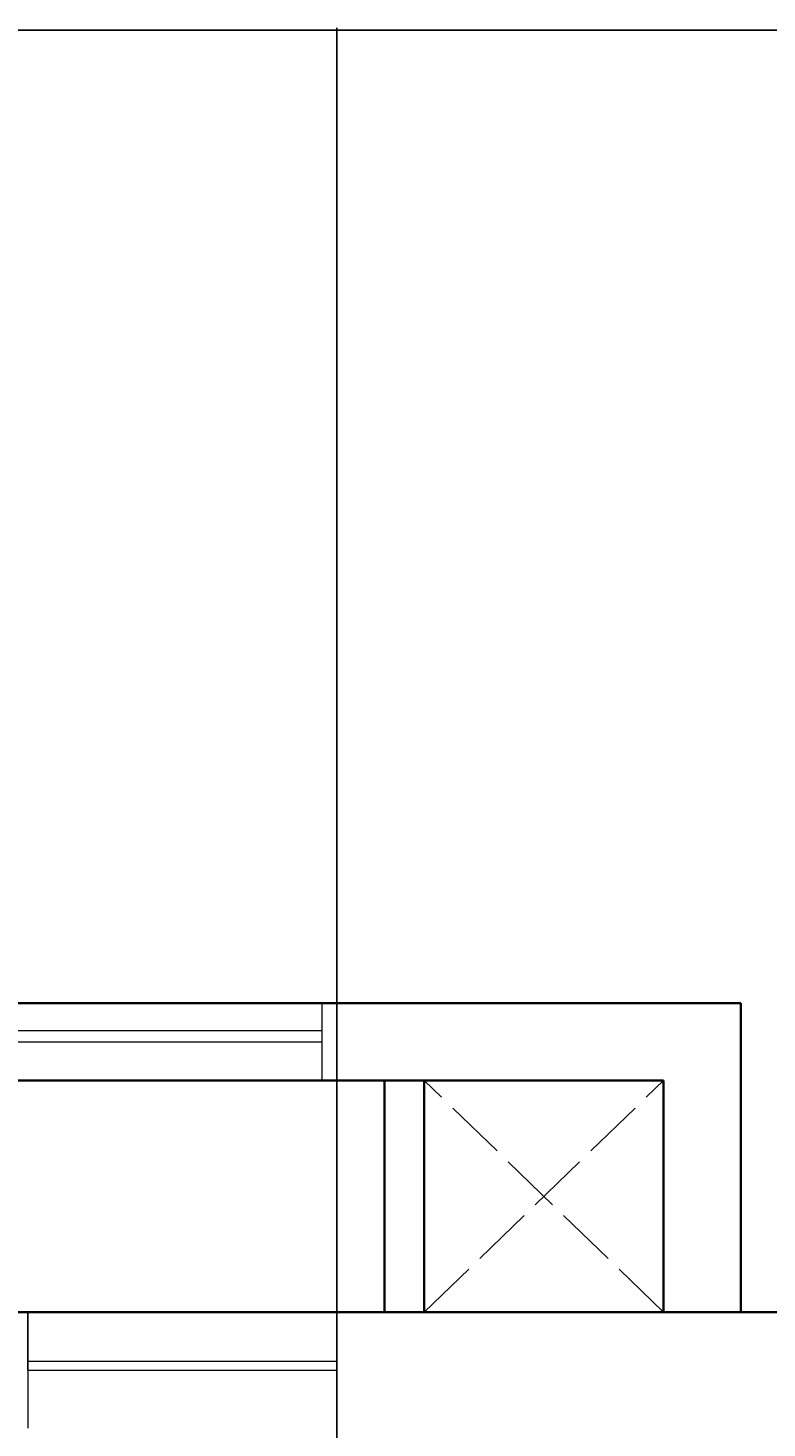
# Model space of a CAD drawing. Units: inches. Extents: x -61 to 1599, y -1316 to 257.
# Tile 144 of 204: x 348 to 406, y 149 to 257. Entities that reach past the tile are written whole.
import ezdxf

# ---------------------------------------------------------------- set-up
doc = ezdxf.new("R2010")
doc.units = ezdxf.units.IN
doc.header["$MEASUREMENT"] = 0
doc.linetypes.add('ACAD_ISO02W100', pattern=[15, 12, -3])
for name, color, linetype, lineweight in [('A-ANNO-DIMS', 2, 'Continuous', 18), ('A-FLOR-OPEN-HIDN', 8, 'ACAD_ISO02W100', 13), ('WALLS', 4, 'Continuous', 35), ('WINDOWS', 220, 'Continuous', 18)]:
    doc.layers.add(name, color=color, linetype=linetype, lineweight=lineweight)
doc.styles.get("Standard").update_dxf_attribs({"font": 'arial.ttf'})
doc.dimstyles.get("Standard").update_dxf_attribs({"dimtxt": 0.18, "dimasz": 0.18, "dimexe": 0.18, "dimexo": 0.0625, "dimgap": 0.09, "dimtad": 0, "dimtih": 1, "dimtoh": 1, "dimdec": 0, "dimzin": 0, "dimdsep": 46, "dimlunit": 3, "dimtxsty": 'Standard', "dimcen": 0.09, "dimadec": 0, "dimazin": 0, "dimtfac": 1, "dimtdec": 0, "dimtofl": 0, "dimtmove": 0, "dimatfit": 3, "dimfxl": 1, "dimtolj": 1, "dimtzin": 0, "dimarcsym": 0})

# ---------------------------------------------------------------- blocks, each defined once
blk = doc.blocks.new('WIN-24IN')
for p, q in [((0, 4.5), (0, 9)), ((0, 9), (0, 0)), ((24, 9), (24, 0)), ((0, 5.19), (24, 5.19)), ((0, 4.5), (24, 4.5))]:
    blk.add_line(p, q)
blk = doc.blocks.new('WIN-51IN')
for p, q in [((0, 0), (0, 6)), ((50.52, 0), (50.52, 6)), ((0, 3.89), (50.52, 3.89)), ((0, 3), (50.52, 3))]:
    blk.add_line(p, q)
blk = doc.blocks.new('*D686')
at = {"layer": 'A-ANNO-DIMS', "color": 0, "lineweight": -2, "transparency": 16777216}
for p, q in [((14.7, 157.74), (14.7, 257.46)), ((14.88, 257.28), (768.35, 257.28)), ((1522.52, 257.28), (769.05, 257.28)), ((1522.7, 157.74), (1522.7, 257.46))]:
    blk.add_line(p, q, dxfattribs=at)
at = {"layer": 'A-ANNO-DIMS', "color": 0, "transparency": 16777216}
for points in [[(14.88, 257.31), (14.88, 257.25), (14.7, 257.28)], [(1522.52, 257.31), (1522.52, 257.25), (1522.7, 257.28)]]:
    blk.add_solid(points, dxfattribs=at)
at = {"layer": 'DEFPOINTS', "color": 0, "transparency": 16777216}
for p in [(1522.7, 257.28), (14.7, 157.68), (1522.7, 157.68)]:
    blk.add_point(p, dxfattribs=at)
at = {"layer": 'A-ANNO-DIMS', "color": 0, "transparency": 16777216, "insert": (768.7, 257.28), "char_height": 0.18, "attachment_point": 5}
blk.add_mtext('\\A1;1508', dxfattribs=at)
blk = doc.blocks.new('*D703')
at = {"layer": 'A-ANNO-DIMS', "color": 0, "lineweight": -2, "transparency": 16777216}
for p, q in [((372.32, -616.88), (372.32, 257.46)), ((372.5, 257.28), (413.7, 257.28)), ((455.65, 257.28), (414.45, 257.28)), ((455.83, -616.88), (455.83, 257.46))]:
    blk.add_line(p, q, dxfattribs=at)
at = {"layer": 'A-ANNO-DIMS', "color": 0, "transparency": 16777216}
for points in [[(372.5, 257.31), (372.5, 257.25), (372.32, 257.28)], [(455.65, 257.31), (455.65, 257.25), (455.83, 257.28)]]:
    blk.add_solid(points, dxfattribs=at)
at = {"layer": 'DEFPOINTS', "color": 0, "transparency": 16777216}
for p in [(455.83, 257.28), (372.32, -616.94), (455.83, -616.94)]:
    blk.add_point(p, dxfattribs=at)
at = {"layer": 'A-ANNO-DIMS', "color": 0, "transparency": 16777216, "insert": (414.08, 257.28), "char_height": 0.18, "attachment_point": 5}
blk.add_mtext('\\A1;83.51', dxfattribs=at)

msp = doc.modelspace()

# ---------------------------------------------------------------- linework, layer by layer
at = {"layer": 'A-FLOR-OPEN-HIDN', "ltscale": 0.4}
for p, q in [((379.1186, 157.6771), (397.7028, 175.6771)), ((397.7028, 157.6771), (379.1186, 175.6771))]:
    msp.add_line(p, q, dxfattribs=at)
at = {"layer": 'WALLS'}
for p, q in [((403.7028, 181.6771), (289.4807, 181.6771)), ((403.7028, 157.6771), (403.7028, 181.6771)), ((397.7028, 175.6771), (295.4807, 175.6771)), ((376.0257, 157.6771), (376.0257, 175.6771)), ((379.1186, 157.6771), (379.1186, 175.6771)), ((397.7028, 157.6771), (397.7028, 175.6771)), ((544.7028, 157.6771), (14.7028, 157.6771))]:
    msp.add_line(p, q, dxfattribs=at)

# ---------------------------------------------------------------- block references
at = {"layer": 'WINDOWS'}
for name, p in [('WIN-51IN', (320.659, 175.677)), ('WIN-24IN', (348.3196, 148.677))]:
    msp.add_blockref(name, p, dxfattribs=at)

# ---------------------------------------------------------------- dimensions: what is measured, and where the dimension line sits
at = {"layer": 'A-ANNO-DIMS'}
for base, p1, p2, override, picture, middle in [((1522.7028, 257.2771), (14.7028, 157.6771), (1522.7028, 157.6771), {"dimdec": 0, "dimlfac": 1, "dimrnd": 0, "dimzin": 0, "dimdsep": 46, "dimlunit": 2}, '*D686', (768.7028, 257.2771)), ((455.8327, 257.2771), (372.3201, -616.9446), (455.8327, -616.9446), {"dimdec": 2, "dimlfac": 1, "dimrnd": 0, "dimzin": 0, "dimdsep": 46, "dimlunit": 2}, '*D703', (414.0764, 257.2771))]:
    dim = msp.add_linear_dim(base=base, p1=p1, p2=p2, dimstyle='Standard', override=override, dxfattribs=at)
    dim.commit()
    dim.dimension.update_dxf_attribs({"geometry": picture, "text_midpoint": middle})

doc.saveas('drawing.dxf')
